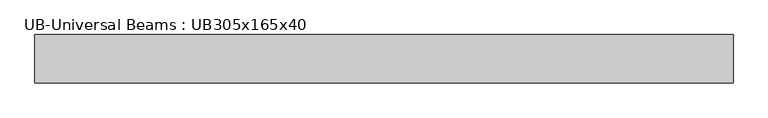
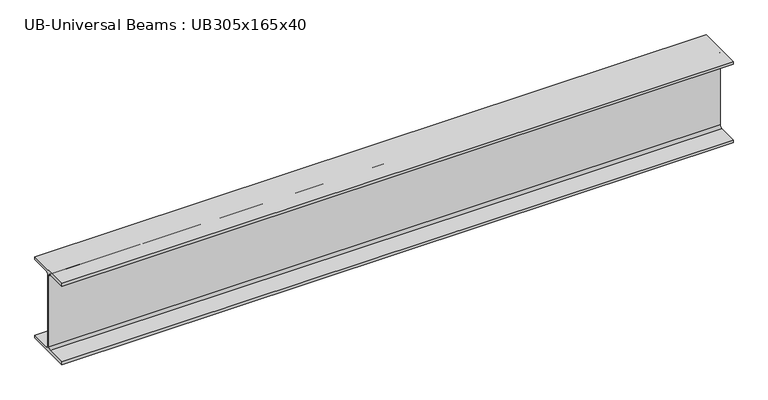
"""IFC4 building model written with IfcOpenShell, lengths in millimetres: beam geometry, UB-Universal Beams : UB305x165x40."""

from ifc_helpers import new_model, si_unit, point, frame, frame_2d, origin, place, context, project, spatial, polyline, circle_curve, trimmed, segment, composite_curve, outline, extrude, source, transform, mapped, element, save


def ub_universal_beams_ub305x165x40_84569ede(model_context):
    return source(origin(), model_context, "Body", "SweptSolid", [
        extrude(outline(composite_curve([segment(polyline([(82.5, -141.5), (82.5, -151.7), (-82.5, -151.7), (-82.5, -141.5), (-11.9, -141.5)]), True, "CONTINUOUS"), segment(trimmed(circle_curve(frame_2d((-11.9, -132.6)), 8.9), [point((-11.9, -141.5))], [point((-3.0, -132.6))], True, "CARTESIAN"), True, "CONTINUOUS"), segment(polyline([(-3.0, -132.6), (-3.0, 132.6)]), True, "CONTINUOUS"), segment(trimmed(circle_curve(frame_2d((-11.9, 132.6)), 8.9), [point((-3.0, 132.6))], [point((-11.9, 141.5))], True, "CARTESIAN"), True, "CONTINUOUS"), segment(polyline([(-11.9, 141.5), (-82.5, 141.5), (-82.5, 151.7), (82.5, 151.7), (82.5, 141.5), (11.9, 141.5)]), True, "CONTINUOUS"), segment(trimmed(circle_curve(frame_2d((11.9, 132.6)), 8.9), [point((11.9, 141.5))], [point((3.0, 132.6))], True, "CARTESIAN"), True, "CONTINUOUS"), segment(polyline([(3.0, 132.6), (3.0, -132.6)]), True, "CONTINUOUS"), segment(trimmed(circle_curve(frame_2d((11.9, -132.6)), 8.9), [point((3.0, -132.6))], [point((11.9, -141.5))], True, "CARTESIAN"), True, "CONTINUOUS"), segment(polyline([(11.9, -141.5), (82.5, -141.5)]), True, "CONTINUOUS")], self_intersect=False)), frame((-1263.55, 0.0, 0.0), z_axis=(1.0, 0.0, 0.0), x_axis=(0.0, 1.0, 0.0)), (0.0, 0.0, 1.0), 2372.4),
    ])


if __name__ == "__main__":
    model = new_model("IFC4")
    model_context = context("Model", 3, world=origin())
    ifc_project = project(units=[si_unit("LENGTHUNIT", "METRE", prefix="MILLI")], contexts=[model_context])
    site = spatial("IfcSite", under=ifc_project)
    building = spatial("IfcBuilding", under=site)
    placement = place(None, origin())
    ub_universal_beams_ub305x165x40_shape = ub_universal_beams_ub305x165x40_84569ede(model_context)
    element("IfcBeam", 1, ObjectType="UB-Universal Beams : UB305x165x40", at=placement, inside=building, context=model_context, shape_type="MappedRepresentation", body=[
        mapped(ub_universal_beams_ub305x165x40_shape, transform((0.0, 0.0, 0.0), x_axis=(1.0, 0.0, 0.0), y_axis=(0.0, 1.0, 0.0), z_axis=(0.0, 0.0, 1.0))),
    ])
    save(model, "model.ifc")

# Revit data of these elements
# Type "UB-Universal Beams : UB305x165x40"
#   Section Name Key = "UB305X165X40"
#   Width = 16.5 cm
#   Web Thickness = 0.6 cm
#   Web Fillet = 0.89 cm
#   Warping Constant = 164000.0 cm⁶
#   Torsional Moment of Inertia = 14.70 cm⁴
#   Section Area = 51.3 cm²
#   Plastic Modulus weak axis = 142.0 cm³
#   Plastic Modulus strong axis = 623.0 cm³
#   Nominal Weight = 40.2999 kgf/m
#   Moment of Inertia weak axis = 764.00 cm⁴
#   Moment of Inertia strong axis = 8503.00 cm⁴
#   Height = 30.34 cm
#   Flange Thickness = 1.02 cm
#   Elastic Modulus weak axis = 92.6 cm³
#   Elastic Modulus strong axis = 560.0 cm³
#   Centroid Vertical = 15.17 cm
#   Centroid Horizontal = 8.25 cm
#   Bolt Spacing = 9.0 cm
#   Length [instance default] = 1500 mm
#   Structural Material [instance default] = Metal - Steel 43-275
#   Type Comments = ""
#   Assembly Code = ""
# Element 1 (IfcBeam, "UB-Universal Beams : UB305x165x40")
#   Materials on its faces: "Metal - Steel 43-275"
# Materials
#   "Metal - Steel 43-275": class "Metal", colour RGB 247 247 247, transparency 0, Cost = 0
